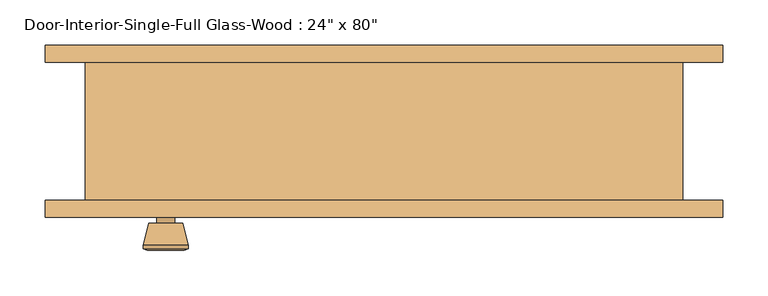
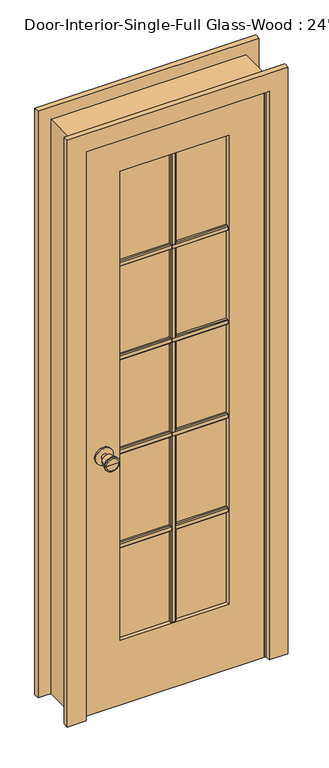
"""IFC4 building model written with IfcOpenShell, lengths in millimetres: door geometry."""

from ifc_helpers import new_model, si_unit, point, frame, frame_2d, origin, place, context, project, spatial, polyline, circle_curve, trimmed, segment, composite_curve, outline, extrude, faceted_brep, source, transform, mapped, element, save
from ifc_brep_helpers import plane_surface, cylinder_surface, revolved_surface, advanced_brep


def door_6d64ae12(model_context):
    return source(origin(), model_context, "Body", "SolidModel", [
        extrude(outline(polyline([(-59.055, 1586.23), (-59.055, 1567.18), (-65.405, 1567.18), (-68.58, 1570.355), (-68.58, 1583.055), (-65.405, 1586.23), (-59.055, 1586.23)])), frame((-184.15, 0.0, 0.0), z_axis=(1.0, 0.0, 0.0), x_axis=(0.0, 1.0, 0.0)), (0.0, 0.0, 1.0), 368.3),
        extrude(outline(polyline([(-59.055, 1249.9975), (-59.055, 1230.9475), (-65.405, 1230.9475), (-68.58, 1234.1225), (-68.58, 1246.8225), (-65.405, 1249.9975), (-59.055, 1249.9975)])), frame((-184.15, 0.0, 0.0), z_axis=(1.0, 0.0, 0.0), x_axis=(0.0, 1.0, 0.0)), (0.0, 0.0, 1.0), 368.3),
        extrude(outline(polyline([(-59.055, 913.765), (-59.055, 894.715), (-65.405, 894.715), (-68.58, 897.89), (-68.58, 910.59), (-65.405, 913.765), (-59.055, 913.765)])), frame((-184.15, 0.0, 0.0), z_axis=(1.0, 0.0, 0.0), x_axis=(0.0, 1.0, 0.0)), (0.0, 0.0, 1.0), 368.3),
        extrude(outline(polyline([(-9.525, -59.055), (9.525, -59.055), (9.525, -65.405), (6.35, -68.58), (-6.35, -68.58), (-9.525, -65.405), (-9.525, -59.055)])), frame((0.0, 0.0, 231.775), z_axis=(0.0, 0.0, 1.0), x_axis=(1.0, 0.0, 0.0)), (0.0, 0.0, 1.0), 1681.1625),
        extrude(outline(polyline([(-59.055, 577.5325), (-59.055, 558.4825), (-65.405, 558.4825), (-68.58, 561.6575), (-68.58, 574.3575), (-65.405, 577.5325), (-59.055, 577.5325)])), frame((-184.15, 0.0, 0.0), z_axis=(1.0, 0.0, 0.0), x_axis=(0.0, 1.0, 0.0)), (0.0, 0.0, 1.0), 368.3),
        extrude(outline(polyline([(-52.07, 1586.23), (-45.72, 1586.23), (-42.545, 1583.055), (-42.545, 1570.355), (-45.72, 1567.18), (-52.07, 1567.18), (-52.07, 1586.23)])), frame((-184.15, 0.0, 0.0), z_axis=(1.0, 0.0, 0.0), x_axis=(0.0, 1.0, 0.0)), (0.0, 0.0, 1.0), 368.3),
        extrude(outline(polyline([(-52.07, 1249.9975), (-45.72, 1249.9975), (-42.545, 1246.8225), (-42.545, 1234.1225), (-45.72, 1230.9475), (-52.07, 1230.9475), (-52.07, 1249.9975)])), frame((-184.15, 0.0, 0.0), z_axis=(1.0, 0.0, 0.0), x_axis=(0.0, 1.0, 0.0)), (0.0, 0.0, 1.0), 368.3),
        extrude(outline(polyline([(-52.07, 913.765), (-45.72, 913.765), (-42.545, 910.59), (-42.545, 897.89), (-45.72, 894.715), (-52.07, 894.715), (-52.07, 913.765)])), frame((-184.15, 0.0, 0.0), z_axis=(1.0, 0.0, 0.0), x_axis=(0.0, 1.0, 0.0)), (0.0, 0.0, 1.0), 368.3),
        extrude(outline(polyline([(-9.525, -52.07), (-9.525, -45.72), (-6.35, -42.545), (6.35, -42.545), (9.525, -45.72), (9.525, -52.07), (-9.525, -52.07)])), frame((0.0, 0.0, 231.775), z_axis=(0.0, 0.0, 1.0), x_axis=(1.0, 0.0, 0.0)), (0.0, 0.0, 1.0), 1681.1625),
        extrude(outline(polyline([(-52.07, 577.5325), (-45.72, 577.5325), (-42.545, 574.3575), (-42.545, 561.6575), (-45.72, 558.4825), (-52.07, 558.4825), (-52.07, 577.5325)])), frame((-184.15, 0.0, 0.0), z_axis=(1.0, 0.0, 0.0), x_axis=(0.0, 1.0, 0.0)), (0.0, 0.0, 1.0), 368.3),
        advanced_brep(
        [(-241.3, -32.1, 914.4), (-251.3, -32.1, 914.4), (-231.3, -32.1, 914.4), (-220.8241324, 16.9, 914.4), (-261.7758676, 16.9, 914.4), (-241.3, 16.9, 914.4), (-216.3, 15.0721319, 914.4), (-266.3, 15.0721319, 914.4), (-216.3, 11.6084537, 914.4), (-266.3, 11.6084537, 914.4), (-222.663764, -13.1, 914.4), (-259.936236, -13.1, 914.4), (-231.3, -13.1, 914.4), (-251.3, -13.1, 914.4)],
        [
            (0, 1),
            (1, 2, circle_curve(frame((-241.3, -32.1, 914.4), z_axis=(0.0, -1.0, 0.0), x_axis=(-1.0, 0.0, 0.0)), 10.0)),
            (2, 0),
            (2, 1, circle_curve(frame((-241.3, -32.1, 914.4), z_axis=(0.0, -1.0, 0.0), x_axis=(-1.0, 0.0, 0.0)), 10.0)),
            (3, 4, circle_curve(frame((-241.3, 16.9, 914.4), z_axis=(0.0, 1.0, 0.0), x_axis=(-1.0, 0.0, 0.0)), 20.4758676)),
            (4, 5),
            (5, 3),
            (4, 3, circle_curve(frame((-241.3, 16.9, 914.4), z_axis=(0.0, 1.0, 0.0), x_axis=(-1.0, 0.0, 0.0)), 20.4758676)),
            (6, 7, circle_curve(frame((-241.3, 15.0721319, 914.4), z_axis=(0.0, 1.0, 0.0), x_axis=(-1.0, 0.0, 0.0)), 25.0)),
            (7, 4),
            (3, 6),
            (7, 6, circle_curve(frame((-241.3, 15.0721319, 914.4), z_axis=(0.0, 1.0, 0.0), x_axis=(-1.0, 0.0, 0.0)), 25.0)),
            (8, 9, circle_curve(frame((-241.3, 11.6084537, 914.4), z_axis=(0.0, 1.0, 0.0), x_axis=(-1.0, 0.0, 0.0)), 25.0)),
            (9, 7),
            (6, 8),
            (9, 8, circle_curve(frame((-241.3, 11.6084537, 914.4), z_axis=(0.0, 1.0, 0.0), x_axis=(-1.0, 0.0, 0.0)), 25.0)),
            (10, 11, circle_curve(frame((-241.3, -13.1, 914.4), z_axis=(0.0, 1.0, 0.0), x_axis=(-1.0, 0.0, 0.0)), 18.636236)),
            (11, 9),
            (8, 10),
            (11, 10, circle_curve(frame((-241.3, -13.1, 914.4), z_axis=(0.0, 1.0, 0.0), x_axis=(-1.0, 0.0, 0.0)), 18.636236)),
            (12, 13, circle_curve(frame((-241.3, -13.1, 914.4), z_axis=(0.0, 1.0, 0.0), x_axis=(-1.0, 0.0, 0.0)), 10.0)),
            (13, 11),
            (10, 12),
            (13, 12, circle_curve(frame((-241.3, -13.1, 914.4), z_axis=(0.0, 1.0, 0.0), x_axis=(-1.0, 0.0, 0.0)), 10.0)),
            (1, 13),
            (12, 2),
        ],
        [
            plane_surface(frame((-241.3, -32.1, 914.4), z_axis=(0.0, -1.0, 0.0), x_axis=(-1.0, 0.0, 0.0))),
            plane_surface(frame((-241.3, 16.9, 914.4), z_axis=(0.0, 1.0, 0.0), x_axis=(-1.0, 0.0, 0.0))),
            revolved_surface(polyline([(-261.7758676, 16.9, 914.4), (-266.3, 15.0721319, 914.4)]), (-241.3, -32.1, 914.4), (0.0, -1.0, 0.0)),
            cylinder_surface(frame((-241.3, -32.1, 914.4), z_axis=(0.0, -1.0, 0.0), x_axis=(-1.0, 0.0, 0.0)), 25.0),
            revolved_surface(polyline([(-266.3, 11.6084537, 914.4), (-259.936236, -13.1, 914.4)]), (-241.3, -32.1, 914.4), (0.0, -1.0, 0.0)),
            plane_surface(frame((-241.3, -13.1, 914.4), z_axis=(0.0, -1.0, 0.0), x_axis=(-1.0, 0.0, 0.0))),
            cylinder_surface(frame((-241.3, -32.1, 914.4), z_axis=(0.0, -1.0, 0.0), x_axis=(-1.0, 0.0, 0.0)), 10.0),
        ],
        [
            (0, [[1, 2, 3]]),
            (0, [[-3, 4, -1]]),
            (1, [[5, 6, 7]]),
            (1, [[8, -7, -6]]),
            (2, [[9, 10, -5, 11]]),
            (2, [[12, -11, -8, -10]]),
            (3, [[13, 14, -9, 15]]),
            (3, [[16, -15, -12, -14]]),
            (4, [[17, 18, -13, 19]]),
            (4, [[20, -19, -16, -18]]),
            (5, [[21, 22, -17, 23]]),
            (5, [[24, -23, -20, -22]]),
            (6, [[-2, 25, -21, 26]]),
            (6, [[-4, -26, -24, -25]]),
        ],
    ),
        extrude(outline(composite_curve([segment(trimmed(circle_curve(frame_2d((914.4, -241.3)), 30.0), [point((914.4, -271.3))], [point((914.4, -211.3))], False, "CARTESIAN"), True, "CONTINUOUS"), segment(trimmed(circle_curve(frame_2d((914.4, -241.3)), 30.0), [point((914.4, -211.3))], [point((914.4, -271.3))], False, "CARTESIAN"), True, "CONTINUOUS")], self_intersect=False)), frame((0.0, -38.1, 0.0), z_axis=(0.0, 1.0, 0.0), x_axis=(0.0, 0.0, 1.0)), (0.0, 0.0, 1.0), 6.0),
        advanced_brep(
        [(-241.3, -79.025, 914.4), (-231.3, -79.025, 914.4), (-251.3, -79.025, 914.4), (-220.8241324, -128.025, 914.4), (-241.3, -128.025, 914.4), (-261.7758676, -128.025, 914.4), (-216.3, -126.1971319, 914.4), (-266.3, -126.1971319, 914.4), (-216.3, -122.7334537, 914.4), (-266.3, -122.7334537, 914.4), (-222.663764, -98.025, 914.4), (-259.936236, -98.025, 914.4), (-231.3, -98.025, 914.4), (-251.3, -98.025, 914.4)],
        [
            (0, 1),
            (1, 2, circle_curve(frame((-241.3, -79.025, 914.4), z_axis=(0.0, 1.0, 0.0), x_axis=(-1.0, 0.0, 0.0)), 10.0)),
            (2, 0),
            (2, 1, circle_curve(frame((-241.3, -79.025, 914.4), z_axis=(0.0, 1.0, 0.0), x_axis=(-1.0, 0.0, 0.0)), 10.0)),
            (3, 4),
            (4, 5),
            (5, 3, circle_curve(frame((-241.3, -128.025, 914.4), z_axis=(0.0, -1.0, 0.0), x_axis=(-1.0, 0.0, 0.0)), 20.4758676)),
            (3, 5, circle_curve(frame((-241.3, -128.025, 914.4), z_axis=(0.0, -1.0, 0.0), x_axis=(-1.0, 0.0, 0.0)), 20.4758676)),
            (6, 3),
            (5, 7),
            (7, 6, circle_curve(frame((-241.3, -126.1971319, 914.4), z_axis=(0.0, -1.0, 0.0), x_axis=(-1.0, 0.0, 0.0)), 25.0)),
            (6, 7, circle_curve(frame((-241.3, -126.1971319, 914.4), z_axis=(0.0, -1.0, 0.0), x_axis=(-1.0, 0.0, 0.0)), 25.0)),
            (8, 6),
            (7, 9),
            (9, 8, circle_curve(frame((-241.3, -122.7334537, 914.4), z_axis=(0.0, -1.0, 0.0), x_axis=(-1.0, 0.0, 0.0)), 25.0)),
            (8, 9, circle_curve(frame((-241.3, -122.7334537, 914.4), z_axis=(0.0, -1.0, 0.0), x_axis=(-1.0, 0.0, 0.0)), 25.0)),
            (10, 8),
            (9, 11),
            (11, 10, circle_curve(frame((-241.3, -98.025, 914.4), z_axis=(0.0, -1.0, 0.0), x_axis=(-1.0, 0.0, 0.0)), 18.636236)),
            (10, 11, circle_curve(frame((-241.3, -98.025, 914.4), z_axis=(0.0, -1.0, 0.0), x_axis=(-1.0, 0.0, 0.0)), 18.636236)),
            (12, 10),
            (11, 13),
            (13, 12, circle_curve(frame((-241.3, -98.025, 914.4), z_axis=(0.0, -1.0, 0.0), x_axis=(-1.0, 0.0, 0.0)), 10.0)),
            (12, 13, circle_curve(frame((-241.3, -98.025, 914.4), z_axis=(0.0, -1.0, 0.0), x_axis=(-1.0, 0.0, 0.0)), 10.0)),
            (1, 12),
            (13, 2),
        ],
        [
            plane_surface(frame((-241.3, -79.025, 914.4), z_axis=(0.0, 1.0, 0.0), x_axis=(-1.0, 0.0, 0.0))),
            plane_surface(frame((-241.3, -128.025, 914.4), z_axis=(0.0, -1.0, 0.0), x_axis=(-1.0, 0.0, 0.0))),
            revolved_surface(polyline([(-261.7758676, -128.025, 914.4), (-266.3, -126.1971319, 914.4)]), (-241.3, -79.025, 914.4), (0.0, 1.0, 0.0)),
            cylinder_surface(frame((-241.3, -79.025, 914.4), z_axis=(0.0, 1.0, 0.0), x_axis=(-1.0, 0.0, 0.0)), 25.0),
            revolved_surface(polyline([(-266.3, -122.7334537, 914.4), (-259.936236, -98.025, 914.4)]), (-241.3, -79.025, 914.4), (0.0, 1.0, 0.0)),
            plane_surface(frame((-241.3, -98.025, 914.4), z_axis=(0.0, 1.0, 0.0), x_axis=(-1.0, 0.0, 0.0))),
            cylinder_surface(frame((-241.3, -79.025, 914.4), z_axis=(0.0, 1.0, 0.0), x_axis=(-1.0, 0.0, 0.0)), 10.0),
        ],
        [
            (0, [[1, 2, 3]]),
            (0, [[-3, 4, -1]]),
            (1, [[5, 6, 7]]),
            (1, [[-6, -5, 8]]),
            (2, [[9, -7, 10, 11]]),
            (2, [[-10, -8, -9, 12]]),
            (3, [[13, -11, 14, 15]]),
            (3, [[-14, -12, -13, 16]]),
            (4, [[17, -15, 18, 19]]),
            (4, [[-18, -16, -17, 20]]),
            (5, [[21, -19, 22, 23]]),
            (5, [[-22, -20, -21, 24]]),
            (6, [[25, -23, 26, -2]]),
            (6, [[-26, -24, -25, -4]]),
        ],
    ),
        extrude(outline(composite_curve([segment(trimmed(circle_curve(frame_2d((914.4, -241.3)), 30.0), [point((914.4, -271.3))], [point((914.4, -211.3))], False, "CARTESIAN"), True, "CONTINUOUS"), segment(trimmed(circle_curve(frame_2d((914.4, -241.3)), 30.0), [point((914.4, -211.3))], [point((914.4, -271.3))], False, "CARTESIAN"), True, "CONTINUOUS")], self_intersect=False)), frame((0.0, -79.025, 0.0), z_axis=(0.0, 1.0, 0.0), x_axis=(0.0, 0.0, 1.0)), (0.0, 0.0, 1.0), 6.0),
        extrude(outline(polyline([(2032.0, -304.8), (0.0, -304.8), (0.0, 304.8), (2032.0, 304.8), (2032.0, -304.8)]), holes=[polyline([(1912.9375, -184.15), (1912.9375, 184.15), (231.775, 184.15), (231.775, -184.15), (1912.9375, -184.15)])]), frame((0.0, -73.025, 0.0), z_axis=(0.0, 1.0, 0.0), x_axis=(0.0, 0.0, 1.0)), (0.0, 0.0, 1.0), 34.925),
        faceted_brep([(330.2, -73.025, 0.0), (304.8, -73.025, 0.0), (304.8, -38.1, 0.0), (292.1, -38.1, 0.0), (292.1, -3.175, 0.0), (304.8, -3.175, 0.0), (304.8, 79.375, 0.0), (330.2, 79.375, 0.0), (330.2, 79.375, 2057.4), (330.2, -73.025, 2057.4), (304.8, 79.375, 2032.0), (-304.8, 79.375, 2032.0), (-304.8, 79.375, 0.0), (-330.2, 79.375, 0.0), (-330.2, 79.375, 2057.4), (304.8, -3.175, 2032.0), (292.1, -3.175, 2019.3), (-292.1, -3.175, 2019.3), (-292.1, -3.175, 0.0), (-304.8, -3.175, 0.0), (-304.8, -3.175, 2032.0), (292.1, -38.1, 2019.3), (304.8, -38.1, 2032.0), (-304.8, -38.1, 2032.0), (-304.8, -38.1, 0.0), (-292.1, -38.1, 0.0), (-292.1, -38.1, 2019.3), (304.8, -73.025, 2032.0), (-330.2, -73.025, 2057.4), (-330.2, -73.025, 0.0), (-304.8, -73.025, 0.0), (-304.8, -73.025, 2032.0)], [[[0, 1, 2, 3, 4, 5, 6, 7]], [[7, 8, 9, 0]], [[6, 10, 11, 12, 13, 14, 8, 7]], [[5, 15, 10, 6]], [[4, 16, 17, 18, 19, 20, 15, 5]], [[3, 21, 16, 4]], [[2, 22, 23, 24, 25, 26, 21, 3]], [[1, 27, 22, 2]], [[0, 9, 28, 29, 30, 31, 27, 1]], [[8, 14, 28, 9]], [[15, 20, 11, 10]], [[21, 26, 17, 16]], [[27, 31, 23, 22]], [[29, 13, 12, 19, 18, 25, 24, 30]], [[14, 13, 29, 28]], [[20, 19, 12, 11]], [[26, 25, 18, 17]], [[31, 30, 24, 23]]]),
        extrude(outline(polyline([(184.15, -52.07), (184.15, -59.055), (-184.15, -59.055), (-184.15, -52.07), (184.15, -52.07)])), frame((0.0, 0.0, 231.775), z_axis=(0.0, 0.0, 1.0), x_axis=(1.0, 0.0, 0.0)), (0.0, 0.0, 1.0), 1681.1625),
        extrude(outline(polyline([(0.0, 374.65), (2101.85, 374.65), (2101.85, -374.65), (0.0, -374.65), (0.0, -311.15), (2038.35, -311.15), (2038.35, 311.15), (0.0, 311.15), (0.0, 374.65)])), frame((0.0, 79.375, 0.0), z_axis=(0.0, 1.0, 0.0), x_axis=(0.0, 0.0, 1.0)), (0.0, 0.0, 1.0), 19.05),
        extrude(outline(polyline([(0.0, 374.65), (2101.85, 374.65), (2101.85, -374.65), (0.0, -374.65), (0.0, -311.15), (2038.35, -311.15), (2038.35, 311.15), (0.0, 311.15), (0.0, 374.65)])), frame((0.0, -92.075, 0.0), z_axis=(0.0, 1.0, 0.0), x_axis=(0.0, 0.0, 1.0)), (0.0, 0.0, 1.0), 19.05),
    ])


if __name__ == "__main__":
    model = new_model("IFC4")
    model_context = context("Model", 3, world=origin())
    ifc_project = project(units=[si_unit("LENGTHUNIT", "METRE", prefix="MILLI")], contexts=[model_context])
    site = spatial("IfcSite", under=ifc_project)
    building = spatial("IfcBuilding", under=site)
    placement = place(None, origin())
    door_shape = door_6d64ae12(model_context)
    element("IfcDoor", 1, ObjectType="Door-Interior-Single-Full Glass-Wood : 24\" x 80\"", at=placement, inside=building, context=model_context, shape_type="MappedRepresentation", body=[
        mapped(door_shape, transform((0.0, 0.0, 0.0), x_axis=(1.0, 0.0, 0.0), y_axis=(0.0, 1.0, 0.0), z_axis=(0.0, 0.0, 1.0))),
    ])
    save(model, "model.ifc")

# Revit data of these elements
# Type "Door-Interior-Single-Full Glass-Wood : 24\" x 80\""
#   Type Mark = "10"
#   Assembly Code = "C1020300"
#   Analytic Construction = "Wood frame with single clear glass"
#   Top Rail = 0' - 4 11/16"
#   Thickness = 0' - 1 3/8"
#   Thermal Resistance (R) = 1.0102 (h·ft²·°F)/BTU
#   Swing Angle [instance default] = 90.00°
#   Stiles = 0' - 4 3/4"
#   Rough Width = 2' - 2"
#   Rough Height = 6' - 9"
#   Height = 6' - 8"
#   Width = 2' - 0"
#   Heat Transfer Coefficient (U) = 0.9900 BTU/(h·ft²·°F)
#   Bottom Rail = 0' - 9 1/8"
#   Show Grill [instance default] = yes
#   Trim Material = Cherry
#   Panel Material = Cherry
#   Frame Material = Cherry
#   Door Handle Material = Aluminum
#   Visual Light Transmittance = 0
#   Solar Heat Gain Coefficient = 0
#   Wall Closure = (empty or 0)
#   Function = (empty or 0)
# Element 1 (IfcDoor, "Door-Interior-Single-Full Glass-Wood : 24\" x 80\"")
#   Materials on its faces: "Cherry", "Aluminum", "Glass"
# Materials
#   "Cherry": class "Wood", colour RGB 226 177 128, transparency 0, Description = "Prunus Serotina", Cost = 0
#   "Aluminum": class "Metal", colour RGB 247 247 247, transparency 0, Description = "Aluminum 6061", Cost = 0
#   "Glass": class "Glass", colour RGB 0 128 192, transparency 0.75, Description = "Soda Lime Glass", Cost = 0
